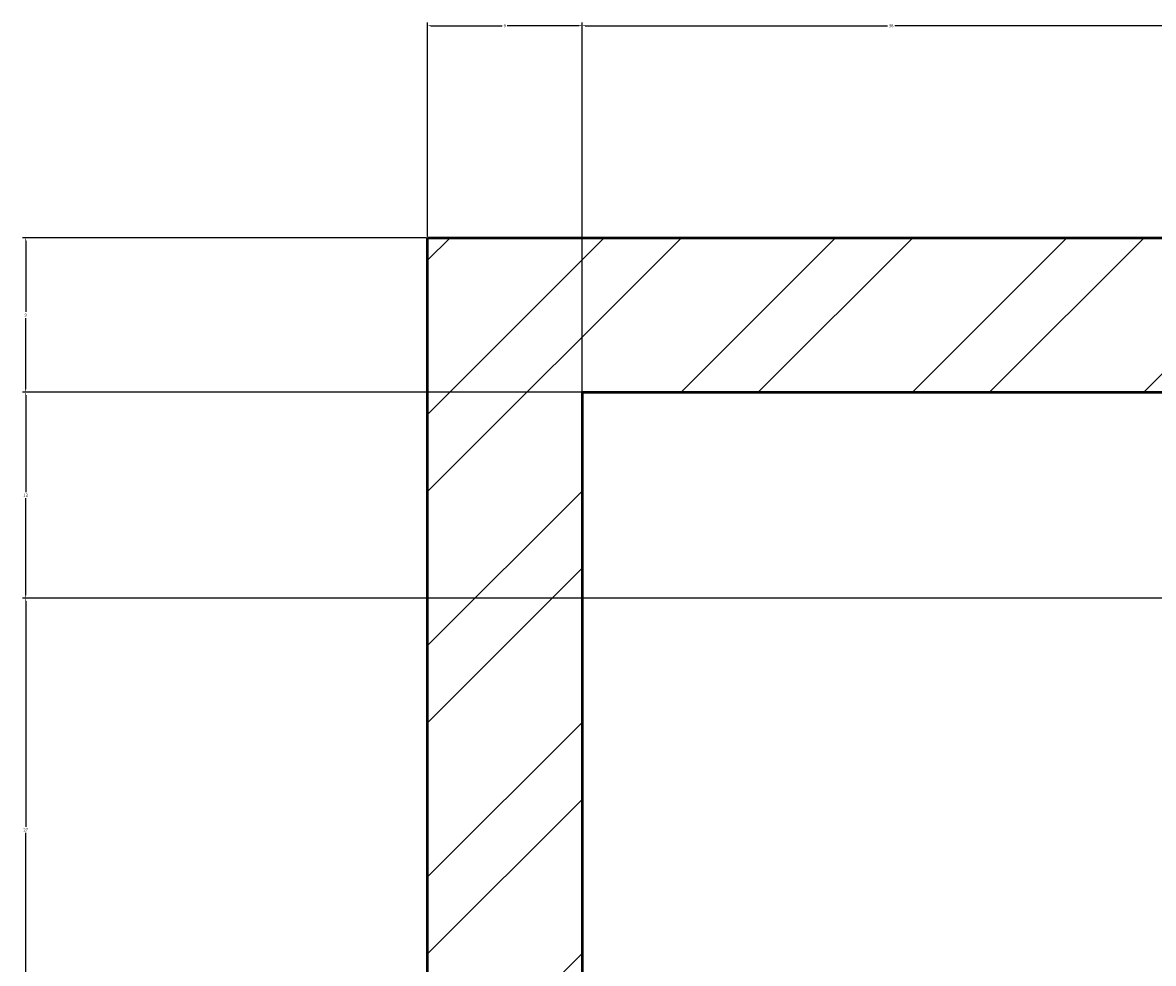
# Model space of a CAD drawing. Units: inches. Extents: x 2812 to 3051, y 1398 to 1659.
# Tile 48 of 65: x 2812 to 2878, y 1605 to 1659. Entities that reach past the tile are written whole.
import ezdxf

# ---------------------------------------------------------------- set-up
doc = ezdxf.new("R2010")
doc.units = ezdxf.units.IN
for name, color, linetype, lineweight in [('A-ANNO-DIMS', 2, 'Continuous', 18), ('S-CONC', 7, 'Continuous', 50), ('S-CONC-PATT', 8, 'Continuous', 18)]:
    doc.layers.add(name, color=color, linetype=linetype, lineweight=lineweight)
doc.styles.get("Standard").update_dxf_attribs({"font": 'arial.ttf'})
doc.dimstyles.get("Standard").update_dxf_attribs({"dimtxt": 0.18, "dimasz": 0.18, "dimexe": 0.18, "dimexo": 0.0625, "dimgap": 0.09, "dimtad": 0, "dimtih": 1, "dimtoh": 1, "dimdec": 4, "dimzin": 0, "dimdsep": 46, "dimtxsty": 'Standard', "dimcen": 0.09, "dimadec": 0, "dimazin": 0, "dimtfac": 1, "dimtdec": 4, "dimtofl": 0, "dimtmove": 0, "dimatfit": 3, "dimfxl": 1, "dimtolj": 1, "dimtzin": 0, "dimarcsym": 0})

# ---------------------------------------------------------------- blocks, each defined once
blk = doc.blocks.new('*D14')
at = {"layer": 'A-ANNO-DIMS', "color": 0, "lineweight": -2, "transparency": 16777216}
for p, q in [((2835.385, 1646.882), (2835.385, 1659.35)), ((2835.565, 1659.17), (2839.736, 1659.17)), ((2844.205, 1659.17), (2840.034, 1659.17)), ((2844.385, 1637.882), (2844.385, 1659.35))]:
    blk.add_line(p, q, dxfattribs=at)
at = {"layer": 'A-ANNO-DIMS', "color": 0, "transparency": 16777216}
for points in [[(2835.565, 1659.2), (2835.565, 1659.14), (2835.385, 1659.17)], [(2844.205, 1659.2), (2844.205, 1659.14), (2844.385, 1659.17)]]:
    blk.add_solid(points, dxfattribs=at)
at = {"layer": 'Defpoints', "color": 0, "transparency": 16777216}
for p in [(2844.385, 1659.17), (2835.385, 1646.82), (2844.385, 1637.82)]:
    blk.add_point(p, dxfattribs=at)
at = {"layer": 'A-ANNO-DIMS', "color": 0, "transparency": 16777216, "insert": (2839.885, 1659.17), "char_height": 0.18, "attachment_point": 5}
blk.add_mtext('\\A1;9', dxfattribs=at)
blk = doc.blocks.new('*D15')
at = {"layer": 'A-ANNO-DIMS', "color": 0, "lineweight": -2, "transparency": 16777216}
for p, q in [((2844.385, 1637.882), (2844.385, 1659.35)), ((2844.565, 1659.17), (2862.166, 1659.17)), ((2880.205, 1659.17), (2862.604, 1659.17)), ((2880.385, 1637.882), (2880.385, 1659.35))]:
    blk.add_line(p, q, dxfattribs=at)
at = {"layer": 'A-ANNO-DIMS', "color": 0, "transparency": 16777216}
for points in [[(2844.565, 1659.2), (2844.565, 1659.14), (2844.385, 1659.17)], [(2880.205, 1659.2), (2880.205, 1659.14), (2880.385, 1659.17)]]:
    blk.add_solid(points, dxfattribs=at)
at = {"layer": 'Defpoints', "color": 0, "transparency": 16777216}
for p in [(2880.385, 1659.17), (2844.385, 1637.82), (2880.385, 1637.82)]:
    blk.add_point(p, dxfattribs=at)
at = {"layer": 'A-ANNO-DIMS', "color": 0, "transparency": 16777216, "insert": (2862.385, 1659.17), "char_height": 0.18, "attachment_point": 5}
blk.add_mtext('\\A1;36', dxfattribs=at)
blk = doc.blocks.new('*D38')
at = {"layer": 'A-ANNO-DIMS', "color": 0, "lineweight": -2, "transparency": 16777216}
for p, q in [((2896.322, 1625.82), (2811.806, 1625.82)), ((2811.986, 1625.64), (2811.986, 1612.5)), ((2811.986, 1599), (2811.986, 1612.14)), ((2910.679, 1598.82), (2811.806, 1598.82))]:
    blk.add_line(p, q, dxfattribs=at)
at = {"layer": 'A-ANNO-DIMS', "color": 0, "transparency": 16777216}
for points in [[(2811.956, 1625.64), (2812.016, 1625.64), (2811.986, 1625.82)], [(2811.956, 1599), (2812.016, 1599), (2811.986, 1598.82)]]:
    blk.add_solid(points, dxfattribs=at)
at = {"layer": 'Defpoints', "color": 0, "transparency": 16777216}
for p in [(2811.986, 1625.82), (2896.385, 1625.82), (2910.742, 1598.82)]:
    blk.add_point(p, dxfattribs=at)
at = {"layer": 'A-ANNO-DIMS', "color": 0, "transparency": 16777216, "insert": (2811.986, 1612.32), "char_height": 0.18, "attachment_point": 5}
blk.add_mtext('\\A1;27', dxfattribs=at)
blk = doc.blocks.new('*D39')
at = {"layer": 'A-ANNO-DIMS', "color": 0, "lineweight": -2, "transparency": 16777216}
for p, q in [((2883.322, 1637.82), (2811.806, 1637.82)), ((2811.986, 1637.64), (2811.986, 1632)), ((2811.986, 1626), (2811.986, 1631.64)), ((2896.322, 1625.82), (2811.806, 1625.82))]:
    blk.add_line(p, q, dxfattribs=at)
at = {"layer": 'A-ANNO-DIMS', "color": 0, "transparency": 16777216}
for points in [[(2811.956, 1637.64), (2812.016, 1637.64), (2811.986, 1637.82)], [(2811.956, 1626), (2812.016, 1626), (2811.986, 1625.82)]]:
    blk.add_solid(points, dxfattribs=at)
at = {"layer": 'Defpoints', "color": 0, "transparency": 16777216}
for p in [(2811.986, 1637.82), (2883.385, 1637.82), (2896.385, 1625.82)]:
    blk.add_point(p, dxfattribs=at)
at = {"layer": 'A-ANNO-DIMS', "color": 0, "transparency": 16777216, "insert": (2811.986, 1631.82), "char_height": 0.18, "attachment_point": 5}
blk.add_mtext('\\A1;12', dxfattribs=at)
blk = doc.blocks.new('*D40')
at = {"layer": 'A-ANNO-DIMS', "color": 0, "lineweight": -2, "transparency": 16777216}
for p, q in [((2835.322, 1646.82), (2811.806, 1646.82)), ((2811.986, 1646.64), (2811.986, 1642.502)), ((2811.986, 1638), (2811.986, 1642.138)), ((2844.322, 1637.82), (2811.806, 1637.82))]:
    blk.add_line(p, q, dxfattribs=at)
at = {"layer": 'A-ANNO-DIMS', "color": 0, "transparency": 16777216}
for points in [[(2811.956, 1646.64), (2812.016, 1646.64), (2811.986, 1646.82)], [(2811.956, 1638), (2812.016, 1638), (2811.986, 1637.82)]]:
    blk.add_solid(points, dxfattribs=at)
at = {"layer": 'Defpoints', "color": 0, "transparency": 16777216}
for p in [(2811.986, 1646.82), (2835.385, 1646.82), (2844.385, 1637.82)]:
    blk.add_point(p, dxfattribs=at)
at = {"layer": 'A-ANNO-DIMS', "color": 0, "transparency": 16777216, "insert": (2811.986, 1642.32), "char_height": 0.18, "attachment_point": 5}
blk.add_mtext('\\A1;9', dxfattribs=at)

msp = doc.modelspace()

# ---------------------------------------------------------------- hatches: boundary and pattern name
at = {"layer": 'S-CONC-PATT'}
h = msp.add_hatch(dxfattribs=at)
h.set_pattern_fill('ANSI32', color=256)
h.paths.add_polyline_path([(3027.3849, 1646.82), (2835.3849, 1646.82), (2835.3849, 1603.2296), (2844.3849, 1603.2296), (2844.3849, 1637.82), (3018.3849, 1637.82), (3018.3849, 1602.5441), (3027.3849, 1602.5441)])
h.paths.add_polyline_path([(2844.3849, 1594.2296), (2835.3849, 1594.2296), (2835.3849, 1550.82), (3027.3849, 1550.82), (3027.3849, 1593.5441), (3018.3849, 1593.5441), (3018.3849, 1559.82), (2844.3849, 1559.82)])
h.paths.add_polyline_path([(2844.3849, 1482.0354), (2835.3849, 1482.0354), (2835.3849, 1463.4959), (2844.3849, 1463.4959)])
h.paths.add_polyline_path([(2844.3849, 1461.4959), (2835.3849, 1461.4959), (2835.3849, 1416.0354), (2844.3849, 1416.0354)])
h.paths.add_polyline_path([(3027.3849, 1482.0354), (3018.3849, 1482.0354), (3018.3849, 1463.2854), (3027.3849, 1463.2854)])
h.paths.add_polyline_path([(3027.3849, 1461.2854), (3018.3849, 1461.2854), (3018.3849, 1416.0354), (3027.3849, 1416.0354)])
h.paths.add_polyline_path([(2961.3849, 1448.4738), (2952.3849, 1448.4738), (2952.3849, 1416.0354), (2961.3849, 1416.0354)])
h.paths.add_polyline_path([(2961.3849, 1462.3026), (2952.3849, 1462.3026), (2952.3849, 1450.4738), (2961.3849, 1450.4738)])
h.paths.add_polyline_path([(2961.3849, 1472.0354), (2952.3849, 1472.0354), (2952.3849, 1462.3026), (2961.3849, 1462.3026)])

# ---------------------------------------------------------------- linework, layer by layer
at = {"layer": 'S-CONC'}
for p, q in [((2835.3849, 1646.82), (3027.3849, 1646.82)), ((2835.3849, 1550.82), (2835.3849, 1646.82)), ((2844.3849, 1637.82), (2844.3849, 1559.82)), ((2844.3849, 1637.82), (3018.3849, 1637.82))]:
    msp.add_line(p, q, dxfattribs=at)

# ---------------------------------------------------------------- dimensions: what is measured, and where the dimension line sits
at = {"layer": 'A-ANNO-DIMS'}
for base, p1, p2, picture, middle in [((2844.3849, 1659.17), (2835.3849, 1646.82), (2844.3849, 1637.82), '*D14', (2839.8849, 1659.17)), ((2880.3849, 1659.17), (2844.3849, 1637.82), (2880.3849, 1637.82), '*D15', (2862.3849, 1659.17))]:
    dim = msp.add_linear_dim(base=base, p1=p1, p2=p2, dimstyle='Standard', override={"dimdec": 0, "dimlfac": 1, "dimrnd": 0, "dimzin": 0, "dimdsep": 46, "dimlunit": 2}, dxfattribs=at)
    dim.commit()
    dim.dimension.update_dxf_attribs({"geometry": picture, "text_midpoint": middle})
for base, p1, p2, picture, middle in [((2811.9855, 1646.82), (2844.3849, 1637.82), (2835.3849, 1646.82), '*D40', (2811.9855, 1642.32)), ((2811.9855, 1637.82), (2896.3849, 1625.82), (2883.3849, 1637.82), '*D39', (2811.9855, 1631.82)), ((2811.9855, 1625.82), (2910.7415, 1598.82), (2896.3849, 1625.82), '*D38', (2811.9855, 1612.32))]:
    dim = msp.add_linear_dim(base=base, p1=p1, p2=p2, angle=90, dimstyle='Standard', override={"dimdec": 0, "dimlfac": 1, "dimrnd": 0, "dimzin": 0, "dimdsep": 46, "dimlunit": 2}, dxfattribs=at)
    dim.commit()
    dim.dimension.update_dxf_attribs({"geometry": picture, "text_midpoint": middle})

doc.saveas('drawing.dxf')
